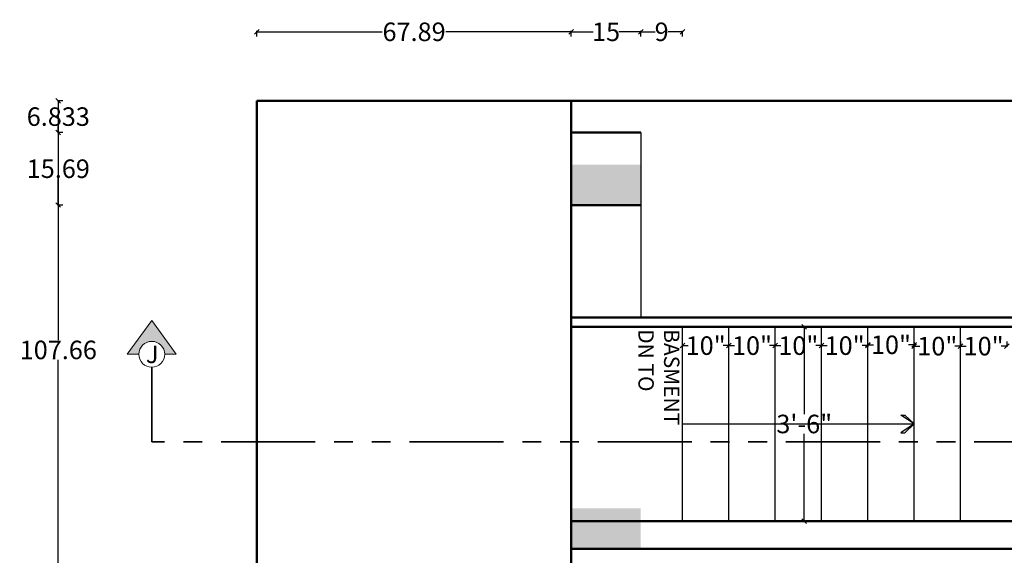
# Model space of a CAD drawing. Units: inches. Extents: x -60 to 284, y -245 to 257.
# Tile 9 of 10: x -52 to 160, y 141 to 257. Entities that reach past the tile are written whole.
import ezdxf

# ---------------------------------------------------------------- set-up
doc = ezdxf.new("R2010")
doc.units = ezdxf.units.IN
doc.header["$LTSCALE"] = 0.8
doc.header["$MEASUREMENT"] = 0
doc.linetypes.add('PHANTOM', pattern=[63.5, 31.75, -6.35, 6.35, -6.35, 6.35, -6.35])
for name, color, linetype, lineweight in [('A-ANNO-DIMS', 2, 'Continuous', 18), ('A-ANNO-SECT', 1, 'PHANTOM', 35), ('A-ANNO-SYMB', 3, 'Continuous', 18), ('A-ANNO-TEXT', 3, 'Continuous', 18), ('A-ANNO-TTLB', 7, 'Continuous', 50), ('A-COLS', 1, 'Continuous', 35), ('A-FLOR-STRS', 4, 'Continuous', 25), ('A-WALL', 7, 'Continuous', 50)]:
    doc.layers.add(name, color=color, linetype=linetype, lineweight=lineweight)
doc.styles.get("Standard").update_dxf_attribs({"font": 'arial.ttf'})
doc.dimstyles.get("Standard").update_dxf_attribs({"dimtxt": 4, "dimasz": 1, "dimexe": 0.18, "dimexo": 0.0625, "dimgap": 0.09, "dimtad": 0, "dimtih": 1, "dimtoh": 1, "dimzin": 0, "dimdsep": 46, "dimlunit": 4, "dimtxsty": 'Standard', "dimblk": 'OBLIQUE', "dimcen": 0.09, "dimadec": 0, "dimazin": 0, "dimtfac": 1, "dimtofl": 0, "dimtmove": 0, "dimatfit": 3, "dimfxl": 1, "dimfxlon": 1, "dimtolj": 1, "dimtzin": 0, "dimarcsym": 0})

# ---------------------------------------------------------------- blocks, each defined once
blk = doc.blocks.new('_Oblique')
at = {"color": 0, "linetype": 'ByBlock', "lineweight": -2}
blk.add_line((-0.5, -0.5), (0.5, 0.5), dxfattribs=at)
blk = doc.blocks.new('*D31')
at = {"layer": 'A-ANNO-DIMS', "color": 0, "lineweight": -2, "ltscale": 0.8, "transparency": 16777216}
for p, q in [((151.01, 187.51), (151.01, 186.33)), ((161.01, 187.51), (161.01, 186.33)), ((151.01, 186.51), (152.26, 186.51)), ((161.01, 186.51), (159.77, 186.51))]:
    blk.add_line(p, q, dxfattribs=at)
at = {"layer": 'Defpoints', "color": 0, "ltscale": 0.8, "transparency": 16777216}
for p in [(151.01, 187.73), (161.01, 187.73), (161.01, 186.51)]:
    blk.add_point(p, dxfattribs=at)
at = {"layer": 'A-ANNO-DIMS', "color": 0, "lineweight": -2, "ltscale": 0.8, "transparency": 16777216, "rotation": 180}
blk.add_blockref('_Oblique', (151.01, 186.51), dxfattribs=at)
at = {"layer": 'A-ANNO-DIMS', "color": 0, "lineweight": -2, "ltscale": 0.8, "transparency": 16777216}
blk.add_blockref('_Oblique', (161.01, 186.51), dxfattribs=at)
at = {"layer": 'A-ANNO-DIMS', "color": 0, "ltscale": 0.8, "transparency": 16777216, "insert": (156.01, 186.51), "char_height": 4, "attachment_point": 5}
blk.add_mtext('\\A1;10"', dxfattribs=at)
blk = doc.blocks.new('*D32')
at = {"layer": 'A-ANNO-DIMS', "color": 0, "lineweight": -2, "ltscale": 0.8, "transparency": 16777216}
for p, q in [((141.01, 187.27), (141.01, 186.33)), ((151.01, 187.51), (151.01, 186.33)), ((141.01, 186.51), (142.26, 186.51)), ((151.01, 186.51), (149.77, 186.51))]:
    blk.add_line(p, q, dxfattribs=at)
at = {"layer": 'Defpoints', "color": 0, "ltscale": 0.8, "transparency": 16777216}
for p in [(141.01, 187.33), (151.01, 187.73), (151.01, 186.51)]:
    blk.add_point(p, dxfattribs=at)
at = {"layer": 'A-ANNO-DIMS', "color": 0, "lineweight": -2, "ltscale": 0.8, "transparency": 16777216, "rotation": 180}
blk.add_blockref('_Oblique', (141.01, 186.51), dxfattribs=at)
at = {"layer": 'A-ANNO-DIMS', "color": 0, "lineweight": -2, "ltscale": 0.8, "transparency": 16777216}
blk.add_blockref('_Oblique', (151.01, 186.51), dxfattribs=at)
at = {"layer": 'A-ANNO-DIMS', "color": 0, "ltscale": 0.8, "transparency": 16777216, "insert": (146.01, 186.51), "char_height": 4, "attachment_point": 5}
blk.add_mtext('\\A1;10"', dxfattribs=at)
blk = doc.blocks.new('*D33')
at = {"layer": 'A-ANNO-DIMS', "color": 0, "lineweight": -2, "ltscale": 0.8, "transparency": 16777216}
for p, q in [((141.01, 187.27), (141.01, 186.62)), ((131.01, 187.02), (131.01, 186.62)), ((131.01, 186.8), (132.26, 186.8)), ((141.01, 186.8), (139.77, 186.8))]:
    blk.add_line(p, q, dxfattribs=at)
at = {"layer": 'Defpoints', "color": 0, "ltscale": 0.8, "transparency": 16777216}
for p in [(131.01, 187.09), (141.01, 187.33), (141.01, 186.8)]:
    blk.add_point(p, dxfattribs=at)
at = {"layer": 'A-ANNO-DIMS', "color": 0, "lineweight": -2, "ltscale": 0.8, "transparency": 16777216, "rotation": 180}
blk.add_blockref('_Oblique', (131.01, 186.8), dxfattribs=at)
at = {"layer": 'A-ANNO-DIMS', "color": 0, "lineweight": -2, "ltscale": 0.8, "transparency": 16777216}
blk.add_blockref('_Oblique', (141.01, 186.8), dxfattribs=at)
at = {"layer": 'A-ANNO-DIMS', "color": 0, "ltscale": 0.8, "transparency": 16777216, "insert": (136.01, 186.8), "char_height": 4, "attachment_point": 5}
blk.add_mtext('\\A1;10"', dxfattribs=at)
blk = doc.blocks.new('*D34')
at = {"layer": 'A-ANNO-DIMS', "color": 0, "lineweight": -2, "ltscale": 0.8, "transparency": 16777216}
for p, q in [((121.01, 186.74), (121.01, 186.44)), ((121.01, 186.62), (122.26, 186.62)), ((131.01, 186.62), (129.77, 186.62)), ((131.01, 187.02), (131.01, 186.44))]:
    blk.add_line(p, q, dxfattribs=at)
at = {"layer": 'Defpoints', "color": 0, "ltscale": 0.8, "transparency": 16777216}
for p in [(131.01, 187.09), (121.01, 186.8), (131.01, 186.62)]:
    blk.add_point(p, dxfattribs=at)
at = {"layer": 'A-ANNO-DIMS', "color": 0, "lineweight": -2, "ltscale": 0.8, "transparency": 16777216, "rotation": 180}
blk.add_blockref('_Oblique', (121.01, 186.62), dxfattribs=at)
at = {"layer": 'A-ANNO-DIMS', "color": 0, "lineweight": -2, "ltscale": 0.8, "transparency": 16777216}
blk.add_blockref('_Oblique', (131.01, 186.62), dxfattribs=at)
at = {"layer": 'A-ANNO-DIMS', "color": 0, "ltscale": 0.8, "transparency": 16777216, "insert": (126.01, 186.62), "char_height": 4, "attachment_point": 5}
blk.add_mtext('\\A1;10"', dxfattribs=at)
blk = doc.blocks.new('*D35')
at = {"layer": 'A-ANNO-DIMS', "color": 0, "lineweight": -2, "ltscale": 0.8, "transparency": 16777216}
for p, q in [((111.01, 186.62), (111.01, 186.8)), ((111.01, 186.62), (112.26, 186.62)), ((121.01, 186.62), (119.77, 186.62)), ((121.01, 186.74), (121.01, 186.44))]:
    blk.add_line(p, q, dxfattribs=at)
at = {"layer": 'Defpoints', "color": 0, "ltscale": 0.8, "transparency": 16777216}
for p in [(111.01, 186.62), (121.01, 186.8), (121.01, 186.62)]:
    blk.add_point(p, dxfattribs=at)
at = {"layer": 'A-ANNO-DIMS', "color": 0, "lineweight": -2, "ltscale": 0.8, "transparency": 16777216, "rotation": 180}
blk.add_blockref('_Oblique', (111.01, 186.62), dxfattribs=at)
at = {"layer": 'A-ANNO-DIMS', "color": 0, "lineweight": -2, "ltscale": 0.8, "transparency": 16777216}
blk.add_blockref('_Oblique', (121.01, 186.62), dxfattribs=at)
at = {"layer": 'A-ANNO-DIMS', "color": 0, "ltscale": 0.8, "transparency": 16777216, "insert": (116.01, 186.62), "char_height": 4, "attachment_point": 5}
blk.add_mtext('\\A1;10"', dxfattribs=at)
blk = doc.blocks.new('*D36')
at = {"layer": 'A-ANNO-DIMS', "color": 0, "lineweight": -2, "ltscale": 0.8, "transparency": 16777216}
for p, q in [((101.01, 186.62), (101.01, 186.8)), ((101.01, 186.62), (102.26, 186.62)), ((111.01, 186.62), (109.77, 186.62)), ((111.01, 186.62), (111.01, 186.8))]:
    blk.add_line(p, q, dxfattribs=at)
at = {"layer": 'Defpoints', "color": 0, "ltscale": 0.8, "transparency": 16777216}
for p in [(101.01, 186.62), (111.01, 186.62), (111.01, 186.62)]:
    blk.add_point(p, dxfattribs=at)
at = {"layer": 'A-ANNO-DIMS', "color": 0, "lineweight": -2, "ltscale": 0.8, "transparency": 16777216, "rotation": 180}
blk.add_blockref('_Oblique', (101.01, 186.62), dxfattribs=at)
at = {"layer": 'A-ANNO-DIMS', "color": 0, "lineweight": -2, "ltscale": 0.8, "transparency": 16777216}
blk.add_blockref('_Oblique', (111.01, 186.62), dxfattribs=at)
at = {"layer": 'A-ANNO-DIMS', "color": 0, "ltscale": 0.8, "transparency": 16777216, "insert": (106.01, 186.62), "char_height": 4, "attachment_point": 5}
blk.add_mtext('\\A1;10"', dxfattribs=at)
blk = doc.blocks.new('*D37')
at = {"layer": 'A-ANNO-DIMS', "color": 0, "lineweight": -2, "ltscale": 0.8, "transparency": 16777216}
for p, q in [((91.01, 186.62), (91.01, 186.8)), ((91.01, 186.62), (92.26, 186.62)), ((101.01, 186.62), (99.77, 186.62)), ((101.01, 186.62), (101.01, 186.8))]:
    blk.add_line(p, q, dxfattribs=at)
at = {"layer": 'Defpoints', "color": 0, "ltscale": 0.8, "transparency": 16777216}
for p in [(91.01, 186.62), (101.01, 186.62), (101.01, 186.62)]:
    blk.add_point(p, dxfattribs=at)
at = {"layer": 'A-ANNO-DIMS', "color": 0, "lineweight": -2, "ltscale": 0.8, "transparency": 16777216, "rotation": 180}
blk.add_blockref('_Oblique', (91.01, 186.62), dxfattribs=at)
at = {"layer": 'A-ANNO-DIMS', "color": 0, "lineweight": -2, "ltscale": 0.8, "transparency": 16777216}
blk.add_blockref('_Oblique', (101.01, 186.62), dxfattribs=at)
at = {"layer": 'A-ANNO-DIMS', "color": 0, "ltscale": 0.8, "transparency": 16777216, "insert": (96.01, 186.62), "char_height": 4, "attachment_point": 5}
blk.add_mtext('\\A1;10"', dxfattribs=at)
blk = doc.blocks.new('*D39')
at = {"layer": 'A-ANNO-DIMS', "color": 0, "lineweight": -2, "ltscale": 0.8, "transparency": 16777216}
for p, q in [((116.29, 190.69), (117.47, 190.69)), ((117.29, 190.69), (117.29, 171.82)), ((117.29, 148.69), (117.29, 167.55)), ((116.29, 148.69), (117.47, 148.69))]:
    blk.add_line(p, q, dxfattribs=at)
at = {"layer": 'Defpoints', "color": 0, "ltscale": 0.8, "transparency": 16777216}
for p in [(114.18, 190.69), (114.18, 148.69), (117.29, 148.69)]:
    blk.add_point(p, dxfattribs=at)
at = {"layer": 'A-ANNO-DIMS', "color": 0, "lineweight": -2, "ltscale": 0.8, "transparency": 16777216}
for p, rotation in [((117.29, 190.69), 90), ((117.29, 148.69), 270)]:
    blk.add_blockref('_Oblique', p, dxfattribs=dict(at, rotation=rotation))
at = {"layer": 'A-ANNO-DIMS', "color": 0, "ltscale": 0.8, "transparency": 16777216, "insert": (117.29, 169.69), "char_height": 4, "attachment_point": 5}
blk.add_mtext('\\A1;3\'-6"', dxfattribs=at)
blk = doc.blocks.new('SECTION-MARK')
at = {"ltscale": 0.8}
for p, q in [((0, 2.79), (5.28, 10.08)), ((10.57, 2.79), (5.28, 10.08)), ((2.5, 2.79), (0, 2.79)), ((8.07, 2.79), (10.57, 2.79))]:
    blk.add_line(p, q, dxfattribs=at)
blk.add_circle((5.28, 2.79), 2.79, dxfattribs=at)
blk = doc.blocks.new('STAIR-ARROW')
at = {"ltscale": 0.8}
for p, q in [((2.04, 3.88), (0, 1.94)), ((0, 1.94), (2.88, 3.86)), ((2.88, 3.86), (2.04, 3.88)), ((50, 1.94), (0, 1.94)), ((0, 1.94), (2.88, 0.03)), ((2.04, 0), (0, 1.94)), ((2.88, 0.03), (2.04, 0))]:
    blk.add_line(p, q, dxfattribs=at)
blk = doc.blocks.new('*D77')
at = {"layer": 'A-ANNO-DIMS', "color": 0, "lineweight": -2, "ltscale": 0.8, "transparency": 16777216}
for p, q in [((-42.73, 239.52), (-43.91, 239.52)), ((-43.73, 239.52), (-43.73, 187.82)), ((-43.73, 131.85), (-43.73, 183.55)), ((-42.73, 131.85), (-43.91, 131.85))]:
    blk.add_line(p, q, dxfattribs=at)
at = {"layer": 'Defpoints', "color": 0, "ltscale": 0.8, "transparency": 16777216}
for p in [(-43.73, 239.52), (-0.88, 239.52), (-0.88, 131.85)]:
    blk.add_point(p, dxfattribs=at)
at = {"layer": 'A-ANNO-DIMS', "color": 0, "lineweight": -2, "ltscale": 0.8, "transparency": 16777216}
for p, rotation in [((-43.73, 239.52), 90), ((-43.73, 131.85), 270)]:
    blk.add_blockref('_Oblique', p, dxfattribs=dict(at, rotation=rotation))
at = {"layer": 'A-ANNO-DIMS', "color": 0, "ltscale": 0.8, "transparency": 16777216, "insert": (-43.73, 185.69), "char_height": 4, "attachment_point": 5}
blk.add_mtext('\\A1;107.66', dxfattribs=at)
blk = doc.blocks.new('*D78')
at = {"layer": 'A-ANNO-DIMS', "color": 0, "lineweight": -2, "ltscale": 0.8, "transparency": 16777216}
for p, q in [((-0.88, 253.42), (-0.88, 254.6)), ((-0.88, 254.42), (26.21, 254.42)), ((67.01, 254.42), (39.92, 254.42)), ((67.01, 253.42), (67.01, 254.6))]:
    blk.add_line(p, q, dxfattribs=at)
at = {"layer": 'Defpoints', "color": 0, "ltscale": 0.8, "transparency": 16777216}
for p in [(67.01, 254.42), (-0.88, 239.52), (67.01, 239.52)]:
    blk.add_point(p, dxfattribs=at)
at = {"layer": 'A-ANNO-DIMS', "color": 0, "lineweight": -2, "ltscale": 0.8, "transparency": 16777216, "rotation": 180}
blk.add_blockref('_Oblique', (-0.88, 254.42), dxfattribs=at)
at = {"layer": 'A-ANNO-DIMS', "color": 0, "lineweight": -2, "ltscale": 0.8, "transparency": 16777216}
blk.add_blockref('_Oblique', (67.01, 254.42), dxfattribs=at)
at = {"layer": 'A-ANNO-DIMS', "color": 0, "ltscale": 0.8, "transparency": 16777216, "insert": (33.07, 254.42), "char_height": 4, "attachment_point": 5}
blk.add_mtext('\\A1;67.89', dxfattribs=at)
blk = doc.blocks.new('*D79')
at = {"layer": 'A-ANNO-DIMS', "color": 0, "lineweight": -2, "ltscale": 0.8, "transparency": 16777216}
for p, q in [((67.01, 253.42), (67.01, 254.6)), ((67.01, 254.42), (71.73, 254.42)), ((82.01, 254.42), (77.3, 254.42)), ((82.01, 253.42), (82.01, 254.6))]:
    blk.add_line(p, q, dxfattribs=at)
at = {"layer": 'Defpoints', "color": 0, "ltscale": 0.8, "transparency": 16777216}
for p in [(82.01, 254.42), (67.01, 232.69), (82.01, 232.69)]:
    blk.add_point(p, dxfattribs=at)
at = {"layer": 'A-ANNO-DIMS', "color": 0, "lineweight": -2, "ltscale": 0.8, "transparency": 16777216, "rotation": 180}
blk.add_blockref('_Oblique', (67.01, 254.42), dxfattribs=at)
at = {"layer": 'A-ANNO-DIMS', "color": 0, "lineweight": -2, "ltscale": 0.8, "transparency": 16777216}
blk.add_blockref('_Oblique', (82.01, 254.42), dxfattribs=at)
at = {"layer": 'A-ANNO-DIMS', "color": 0, "ltscale": 0.8, "transparency": 16777216, "insert": (74.51, 254.42), "char_height": 4, "attachment_point": 5}
blk.add_mtext('\\A1;15', dxfattribs=at)
blk = doc.blocks.new('*D80')
at = {"layer": 'A-ANNO-DIMS', "color": 0, "lineweight": -2, "ltscale": 0.8, "transparency": 16777216}
for p, q in [((82.01, 253.42), (82.01, 254.6)), ((82.01, 254.42), (85.11, 254.42)), ((91.01, 254.42), (87.92, 254.42)), ((91.01, 253.42), (91.01, 254.6))]:
    blk.add_line(p, q, dxfattribs=at)
at = {"layer": 'Defpoints', "color": 0, "ltscale": 0.8, "transparency": 16777216}
for p in [(91.01, 254.42), (82.01, 217), (91.01, 190.69)]:
    blk.add_point(p, dxfattribs=at)
at = {"layer": 'A-ANNO-DIMS', "color": 0, "lineweight": -2, "ltscale": 0.8, "transparency": 16777216, "rotation": 180}
blk.add_blockref('_Oblique', (82.01, 254.42), dxfattribs=at)
at = {"layer": 'A-ANNO-DIMS', "color": 0, "lineweight": -2, "ltscale": 0.8, "transparency": 16777216}
blk.add_blockref('_Oblique', (91.01, 254.42), dxfattribs=at)
at = {"layer": 'A-ANNO-DIMS', "color": 0, "ltscale": 0.8, "transparency": 16777216, "insert": (86.51, 254.42), "char_height": 4, "attachment_point": 5}
blk.add_mtext('\\A1;9', dxfattribs=at)
blk = doc.blocks.new('*D87')
at = {"layer": 'A-ANNO-DIMS', "color": 0, "lineweight": -2, "ltscale": 0.8, "transparency": 16777216}
for p, q in [((-42.73, 232.69), (-43.91, 232.69)), ((-43.73, 232.69), (-43.73, 226.97)), ((-43.73, 217), (-43.73, 222.71)), ((-42.73, 217), (-43.91, 217))]:
    blk.add_line(p, q, dxfattribs=at)
at = {"layer": 'Defpoints', "color": 0, "ltscale": 0.8, "transparency": 16777216}
for p in [(-43.73, 232.69), (82.01, 232.69), (82.01, 217)]:
    blk.add_point(p, dxfattribs=at)
at = {"layer": 'A-ANNO-DIMS', "color": 0, "lineweight": -2, "ltscale": 0.8, "transparency": 16777216}
for p, rotation in [((-43.73, 232.69), 90), ((-43.73, 217), 270)]:
    blk.add_blockref('_Oblique', p, dxfattribs=dict(at, rotation=rotation))
at = {"layer": 'A-ANNO-DIMS', "color": 0, "ltscale": 0.8, "transparency": 16777216, "insert": (-43.73, 224.84), "char_height": 4, "attachment_point": 5}
blk.add_mtext('\\A1;15.69', dxfattribs=at)
blk = doc.blocks.new('*D88')
at = {"layer": 'A-ANNO-DIMS', "color": 0, "lineweight": -2, "ltscale": 0.8, "transparency": 16777216}
for p, q in [((-42.73, 239.52), (-43.91, 239.52)), ((-43.73, 239.52), (-43.73, 238.24)), ((-43.73, 232.69), (-43.73, 233.97)), ((-42.73, 232.69), (-43.91, 232.69))]:
    blk.add_line(p, q, dxfattribs=at)
at = {"layer": 'Defpoints', "color": 0, "ltscale": 0.8, "transparency": 16777216}
for p in [(-43.73, 239.52), (67.01, 239.52), (67.01, 232.69)]:
    blk.add_point(p, dxfattribs=at)
at = {"layer": 'A-ANNO-DIMS', "color": 0, "lineweight": -2, "ltscale": 0.8, "transparency": 16777216}
for p, rotation in [((-43.73, 239.52), 90), ((-43.73, 232.69), 270)]:
    blk.add_blockref('_Oblique', p, dxfattribs=dict(at, rotation=rotation))
at = {"layer": 'A-ANNO-DIMS', "color": 0, "ltscale": 0.8, "transparency": 16777216, "insert": (-43.73, 236.1), "char_height": 4, "attachment_point": 5}
blk.add_mtext('\\A1;6.833', dxfattribs=at)

msp = doc.modelspace()

# ---------------------------------------------------------------- hatches: boundary and pattern name
at = {"layer": 'A-ANNO-SYMB', "ltscale": 0.8}
h = msp.add_hatch(color=256, dxfattribs=at)
h.dxf.hatch_style = 1
h.paths.add_polyline_path([(-28.8318, 184.7402), (-26.3347, 184.7402, -1), (-20.7631, 184.7402), (-18.2661, 184.7402), (-23.5489, 192.0356)])
at = {"layer": 'A-COLS', "ltscale": 0.8}
h = msp.add_hatch(color=256, dxfattribs=at)
h.dxf.hatch_style = 1
h.paths.add_polyline_path([(82.0139, 225.7452), (67.0139, 225.7452), (67.0139, 216.7452), (82.0139, 216.7452)])
h = msp.add_hatch(color=256, dxfattribs=at)
h.dxf.hatch_style = 1
h.paths.add_polyline_path([(82.0139, 151.4349), (67.0139, 151.4349), (67.0139, 142.4349), (82.0139, 142.4349)])

# ---------------------------------------------------------------- linework, layer by layer
at = {"layer": 'A-ANNO-SECT', "ltscale": 0.8}
for p in [(-23.5489, 181.9544), (255.5807, 165.8004)]:
    msp.add_line(p, (-23.5489, 165.8004), dxfattribs=at)
at = {"layer": 'A-ANNO-TTLB', "ltscale": 0.8}
msp.add_lwpolyline([(-0.8787, 239.5184), (230.4297, 239.5184), (230.4297, 131.8542), (-0.8787, 131.8542)], close=True, dxfattribs=at)
at = {"layer": 'A-FLOR-STRS', "ltscale": 0.8}
for p, q in [((67.0139, 190.6856), (67.0139, 232.6856)), ((82.0139, 232.6856), (82.0139, 192.6856)), ((91.0139, 148.6856), (91.0139, 190.6856)), ((101.0139, 148.6856), (101.0139, 190.6856)), ((111.0139, 148.6856), (111.0139, 190.6856)), ((121.0139, 148.6856), (121.0139, 190.6856)), ((131.0139, 148.6856), (131.0139, 190.6856)), ((141.0139, 148.6856), (141.0139, 190.6856)), ((151.0139, 148.6856), (151.0139, 190.6856))]:
    msp.add_line(p, q, dxfattribs=at)
at = {"layer": 'A-WALL', "ltscale": 0.8}
for p, q in [((67.0139, 131.8542), (67.0139, 239.5184)), ((67.0139, 232.6856), (82.0139, 232.6856)), ((82.0139, 216.996), (67.0139, 216.996)), ((67.0139, 192.6856), (211.0139, 192.6856)), ((67.0139, 190.6856), (211.0139, 190.6856)), ((82.0139, 148.6856), (67.0139, 148.6856)), ((82.0139, 148.6856), (230.4297, 148.6856)), ((82.0139, 142.6856), (67.0139, 142.6856)), ((82.0139, 142.6856), (230.4297, 142.6856))]:
    msp.add_line(p, q, dxfattribs=at)

# ---------------------------------------------------------------- block references
at = {"layer": 'A-ANNO-SYMB'}
msp.add_blockref('SECTION-MARK', (-28.8316, 181.9544), dxfattribs=at)
at = {"layer": 'A-FLOR-STRS', "rotation": 180}
msp.add_blockref('STAIR-ARROW', (141.0138, 171.6273), dxfattribs=at)

# ---------------------------------------------------------------- texts
at = {"layer": 'A-ANNO-TEXT', "ltscale": 0.8, "insert": (90.3366, 190.1646), "char_height": 3.316205, "attachment_point": 1, "rotation": 270}
msp.add_mtext_dynamic_manual_height_columns('\\A1;BASMENT\\PDN TO', width=69.138891, gutter_width=0.3685, heights=[0], dxfattribs=at)
at = {"layer": 'A-ANNO-TEXT', "ltscale": 0.8, "insert": (-24.8197, 186.6092), "char_height": 3.7545, "attachment_point": 1}
msp.add_mtext_dynamic_manual_height_columns('J', width=2.355391, gutter_width=0.4172, heights=[0], dxfattribs=at)

# ---------------------------------------------------------------- dimensions: what is measured, and where the dimension line sits
at = {"layer": 'A-ANNO-DIMS', "ltscale": 0.8}
for base, p1, p2, override, picture, middle in [((67.0139, 254.4184), (-0.8787, 239.5184), (67.0139, 239.5184), {"dimdec": 2, "dimlfac": 1, "dimrnd": 0, "dimzin": 0, "dimdsep": 46, "dimlunit": 2}, '*D78', (33.0676, 254.4184)), ((82.0139, 254.4184), (67.0139, 232.6856), (82.0139, 232.6856), {"dimdec": 0, "dimlfac": 1, "dimrnd": 0, "dimzin": 0, "dimdsep": 46, "dimlunit": 2}, '*D79', (74.5139, 254.4184)), ((91.0139, 254.4184), (82.0139, 216.996), (91.0139, 190.6856), {"dimdec": 0, "dimlfac": 1, "dimrnd": 0, "dimzin": 0, "dimdsep": 46, "dimlunit": 2}, '*D80', (86.5139, 254.4184)), ((101.0139, 186.6175), (91.0139, 186.6175), (101.0139, 186.6175), {"dimclrd": 0, "dimclre": 0, "dimclrt": 0}, '*D37', (96.0139, 186.6175)), ((111.0139, 186.6175), (101.0139, 186.6175), (111.0139, 186.6175), {"dimclrd": 0, "dimclre": 0, "dimclrt": 0}, '*D36', (106.0139, 186.6175)), ((121.0139, 186.6175), (111.0139, 186.6175), (121.0139, 186.7975), {"dimclrd": 0, "dimclre": 0, "dimclrt": 0}, '*D35', (116.0139, 186.6175)), ((131.0139, 186.6175), (121.0139, 186.7975), (131.0139, 187.0862), {"dimclrd": 0, "dimclre": 0, "dimclrt": 0}, '*D34', (126.0139, 186.6175)), ((141.0139, 186.7975), (131.0139, 187.0862), (141.0139, 187.3292), {"dimclrd": 0, "dimclre": 0, "dimclrt": 0}, '*D33', (136.0139, 186.7975)), ((151.0139, 186.5084), (141.0139, 187.3292), (151.0139, 187.7334), {"dimclrd": 0, "dimclre": 0, "dimclrt": 0}, '*D32', (146.0139, 186.5084)), ((161.0139, 186.5084), (151.0139, 187.7334), (161.0139, 187.7334), {"dimclrd": 0, "dimclre": 0, "dimclrt": 0}, '*D31', (156.0139, 186.5084))]:
    dim = msp.add_linear_dim(base=base, p1=p1, p2=p2, dimstyle='Standard', override=override, dxfattribs=at)
    dim.commit()
    dim.dimension.update_dxf_attribs({"geometry": picture, "text_midpoint": middle})
for base, p1, p2, override, picture, middle in [((-43.7318, 239.5184), (-0.8787, 131.8542), (-0.8787, 239.5184), {"dimdec": 2, "dimlfac": 1, "dimrnd": 0, "dimzin": 0, "dimdsep": 46, "dimlunit": 2}, '*D77', (-43.7318, 185.6863)), ((-43.7318, 239.5184), (67.0139, 232.6856), (67.0139, 239.5184), {"dimdec": 3, "dimlfac": 1, "dimrnd": 0, "dimzin": 0, "dimdsep": 46, "dimlunit": 2}, '*D88', (-43.7318, 236.102)), ((-43.7318, 232.6856), (82.0139, 216.996), (82.0139, 232.6856), {"dimdec": 2, "dimlfac": 1, "dimrnd": 0, "dimzin": 0, "dimdsep": 46, "dimlunit": 2}, '*D87', (-43.7318, 224.8408)), ((117.2945, 148.6856), (114.1823, 190.6856), (114.1823, 148.6856), {"dimclrd": 0, "dimclre": 0, "dimclrt": 0}, '*D39', (117.2945, 169.6856))]:
    dim = msp.add_linear_dim(base=base, p1=p1, p2=p2, angle=90, dimstyle='Standard', override=override, dxfattribs=at)
    dim.commit()
    dim.dimension.update_dxf_attribs({"geometry": picture, "text_midpoint": middle})

doc.saveas('drawing.dxf')
